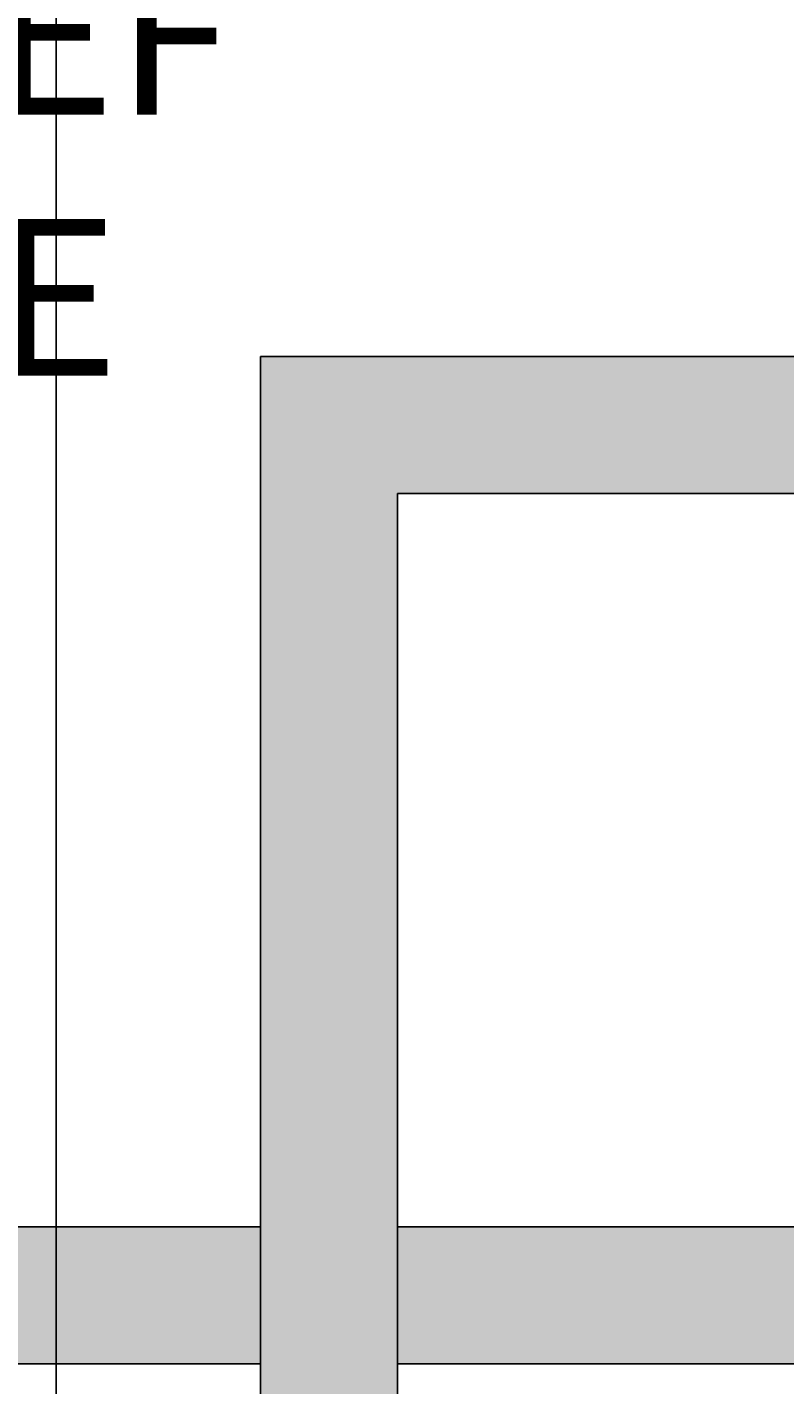
# Model space of a CAD drawing. Units: millimetres. Extents: x -11 to 280, y -4 to 208.
# Tile 29 of 55: x 150 to 170, y 54 to 88. Entities that reach past the tile are written whole.
import ezdxf

# ---------------------------------------------------------------- set-up
doc = ezdxf.new("R2010")
doc.units = ezdxf.units.MM
for name, color, linetype, lineweight in [('M-ANNO-TEXT', 7, 'Continuous', 18), ('M-DIMS', 2, 'Continuous', 18), ('M-HYDR-RETN', 7, 'Continuous', 25)]:
    doc.layers.add(name, color=color, linetype=linetype, lineweight=lineweight)
doc.layers.add('M-HYDR-RETN-PATT', color=114, linetype='Continuous', lineweight=13, true_color=0x139b48)
doc.styles.get("Standard").update_dxf_attribs({"font": 'arial.ttf'})
doc.dimstyles.get("Standard").update_dxf_attribs({"dimtxt": 0.18, "dimasz": 0.18, "dimexe": 0.18, "dimexo": 0.0625, "dimgap": 0.09, "dimtad": 0, "dimtih": 1, "dimtoh": 1, "dimdec": 4, "dimzin": 0, "dimdsep": 46, "dimtxsty": 'Standard', "dimcen": 0.09, "dimadec": 0, "dimazin": 0, "dimtfac": 1, "dimtdec": 4, "dimtofl": 0, "dimtmove": 0, "dimatfit": 3, "dimfxl": 1, "dimtolj": 1, "dimtzin": 0, "dimarcsym": 0})

# ---------------------------------------------------------------- blocks, each defined once
blk = doc.blocks.new('*D4')
at = {"layer": 'Defpoints', "color": 0, "transparency": 16777216}
for p in [(4.763, 84.426), (266.035, 51.733), (266.035, -3.415)]:
    blk.add_point(p, dxfattribs=at)
at = {"layer": 'M-DIMS', "color": 0, "lineweight": -2, "transparency": 16777216}
for p, q in [((4.763, 84.364), (4.763, -3.595)), ((266.035, 51.67), (266.035, -3.595)), ((4.943, -3.415), (134.934, -3.415)), ((265.855, -3.415), (135.864, -3.415))]:
    blk.add_line(p, q, dxfattribs=at)
at = {"layer": 'M-DIMS', "color": 0, "transparency": 16777216}
for points in [[(4.943, -3.385), (4.943, -3.445), (4.763, -3.415)], [(265.855, -3.385), (265.855, -3.445), (266.035, -3.415)]]:
    blk.add_solid(points, dxfattribs=at)
at = {"layer": 'M-DIMS', "color": 0, "transparency": 16777216, "insert": (135.399, -3.415), "char_height": 0.18, "attachment_point": 5}
blk.add_mtext('\\A1;261.27', dxfattribs=at)
blk = doc.blocks.new('*D5')
at = {"layer": 'Defpoints', "color": 0, "transparency": 16777216}
for p in [(24.759, 192.645), (-10.087, 11.435), (261.686, 11.435)]:
    blk.add_point(p, dxfattribs=at)
at = {"layer": 'M-DIMS', "color": 0, "lineweight": -2, "transparency": 16777216}
for p, q in [((24.696, 192.645), (-10.267, 192.645)), ((-10.087, 192.465), (-10.087, 102.222)), ((-10.087, 11.615), (-10.087, 101.858)), ((261.624, 11.435), (-10.267, 11.435))]:
    blk.add_line(p, q, dxfattribs=at)
at = {"layer": 'M-DIMS', "color": 0, "transparency": 16777216}
for points in [[(-10.117, 192.465), (-10.057, 192.465), (-10.087, 192.645)], [(-10.117, 11.615), (-10.057, 11.615), (-10.087, 11.435)]]:
    blk.add_solid(points, dxfattribs=at)
at = {"layer": 'M-DIMS', "color": 0, "transparency": 16777216, "insert": (-10.087, 102.04), "char_height": 0.18, "attachment_point": 5}
blk.add_mtext('\\A1;181.2', dxfattribs=at)
blk = doc.blocks.new('*D18')
at = {"layer": 'Defpoints', "color": 0, "transparency": 16777216}
for p in [(173.804, 207.495), (173.804, 65.064), (151.022, 43.599)]:
    blk.add_point(p, dxfattribs=at)
at = {"layer": 'M-DIMS', "color": 0, "lineweight": -2, "transparency": 16777216}
for p, q in [((151.022, 43.662), (151.022, 207.675)), ((151.202, 207.495), (162.017, 207.495)), ((173.624, 207.495), (162.808, 207.495)), ((173.804, 65.126), (173.804, 207.675))]:
    blk.add_line(p, q, dxfattribs=at)
at = {"layer": 'M-DIMS', "color": 0, "transparency": 16777216}
for points in [[(151.202, 207.525), (151.202, 207.465), (151.022, 207.495)], [(173.624, 207.525), (173.624, 207.465), (173.804, 207.495)]]:
    blk.add_solid(points, dxfattribs=at)
at = {"layer": 'M-DIMS', "color": 0, "transparency": 16777216, "insert": (162.413, 207.495), "char_height": 0.18, "attachment_point": 5}
blk.add_mtext('\\A1;22.78', dxfattribs=at)
blk = doc.blocks.new('*D20')
at = {"layer": 'Defpoints', "color": 0, "transparency": 16777216}
for p in [(231.68, 207.495), (151.022, 43.599), (231.68, 43.599)]:
    blk.add_point(p, dxfattribs=at)
at = {"layer": 'M-DIMS', "color": 0, "lineweight": -2, "transparency": 16777216}
for p, q in [((151.022, 43.662), (151.022, 207.675)), ((151.202, 207.495), (190.957, 207.495)), ((231.5, 207.495), (191.745, 207.495)), ((231.68, 43.662), (231.68, 207.675))]:
    blk.add_line(p, q, dxfattribs=at)
at = {"layer": 'M-DIMS', "color": 0, "transparency": 16777216}
for points in [[(151.202, 207.525), (151.202, 207.465), (151.022, 207.495)], [(231.5, 207.525), (231.5, 207.465), (231.68, 207.495)]]:
    blk.add_solid(points, dxfattribs=at)
at = {"layer": 'M-DIMS', "color": 0, "transparency": 16777216, "insert": (191.351, 207.495), "char_height": 0.18, "attachment_point": 5}
blk.add_mtext('\\A1;80.66', dxfattribs=at)

msp = doc.modelspace()

# ---------------------------------------------------------------- hatches: boundary and pattern name
at = {"layer": 'M-HYDR-RETN-PATT'}
h = msp.add_hatch(color=256, dxfattribs=at)
h.set_gradient(color1=(19, 155, 72), color2=(19, 155, 72), tint=1)
h.paths.add_polyline_path([(17.9701, 159.0814), (29.2015, 159.0814), (29.2015, 162.5814), (14.4701, 162.5814), (14.4701, 98.0213), (17.9701, 98.0213)])
h.paths.add_polyline_path([(17.9701, 84.4261), (14.4701, 84.4261), (14.4701, 54.3099), (156.2446, 54.3099), (156.2446, 57.8099), (17.9701, 57.8099)])
h.paths.add_polyline_path([(120.5137, 74.3991), (17.9701, 74.3991), (17.9701, 70.8991), (120.5137, 70.8991)], flags=17)
h.paths.add_polyline_path([(184.7092, 75.04, 0.4142136), (179.7092, 80.04), (156.2446, 80.04), (156.2446, 57.8099), (156.2446, 54.3099), (156.2446, 43.5991), (159.7446, 43.5991), (159.7446, 57.8099), (159.7446, 76.54), (176.2092, 76.54, -0.4142136), (181.2092, 71.54), (181.2092, 57.8099), (159.7446, 57.8099), (159.7446, 54.3099), (184.7092, 54.3099)])

# ---------------------------------------------------------------- linework, layer by layer
at = {"layer": 'M-HYDR-RETN'}
for points in [[(14.4701, 84.4261), (14.4701, 54.3099), (156.2446, 54.3099)], [(17.9701, 84.4261), (17.9701, 57.8099), (156.2446, 57.8099)], [(156.2446, 57.8099), (156.2446, 41.5991)], [(159.7446, 57.8099), (159.7446, 41.5991)]]:
    msp.add_lwpolyline(points, dxfattribs=at)
msp.add_lwpolyline([(159.7446, 54.3099), (184.7092, 54.3099), (184.7092, 75.04, 0.4142136), (179.7092, 80.04), (156.2446, 80.04), (156.2446, 57.8099)], format="xyb", dxfattribs=at)
msp.add_lwpolyline([(159.7446, 57.8099), (181.2092, 57.8099), (181.2092, 71.54, 0.4142136), (176.2092, 76.54), (159.7446, 76.54)], format="xyb", close=True, dxfattribs=at)

# ---------------------------------------------------------------- texts
at = {"layer": 'M-ANNO-TEXT', "insert": (136.8574, 96.8862), "char_height": 4, "attachment_point": 1}
msp.add_mtext_dynamic_manual_height_columns('PRESSURE\\P RELIEF\\PVALVE', width=63.617875, gutter_width=12.5, heights=[0], dxfattribs=at)

# ---------------------------------------------------------------- dimensions: what is measured, and where the dimension line sits
at = {"layer": 'M-DIMS'}
for base, p1, p2, picture, middle in [((173.8038, 207.495), (151.0217, 43.5991), (173.8038, 65.0638), '*D18', (162.4127, 207.495)), ((231.6803, 207.495), (151.0217, 43.5991), (231.6803, 43.5991), '*D20', (191.351, 207.495)), ((266.0352, -3.4154), (4.7635, 84.4261), (266.0352, 51.7328), '*D4', (135.3993, -3.4154))]:
    dim = msp.add_linear_dim(base=base, p1=p1, p2=p2, dimstyle='Standard', override={"dimdec": 2, "dimlfac": 1, "dimrnd": 0, "dimzin": 0, "dimdsep": 46, "dimlunit": 2}, dxfattribs=at)
    dim.commit()
    dim.dimension.update_dxf_attribs({"geometry": picture, "text_midpoint": middle})
dim = msp.add_linear_dim(base=(-10.0865, 11.4346), p1=(24.7588, 192.645), p2=(261.6863, 11.4346), angle=90, dimstyle='Standard', override={"dimdec": 1, "dimlfac": 1, "dimrnd": 0, "dimzin": 0, "dimdsep": 46, "dimlunit": 2}, dxfattribs=at)
dim.commit()
dim.dimension.update_dxf_attribs({"geometry": '*D5', "text_midpoint": (-10.0865, 102.0398)})

doc.saveas('drawing.dxf')
